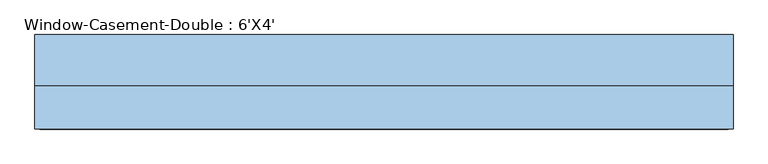
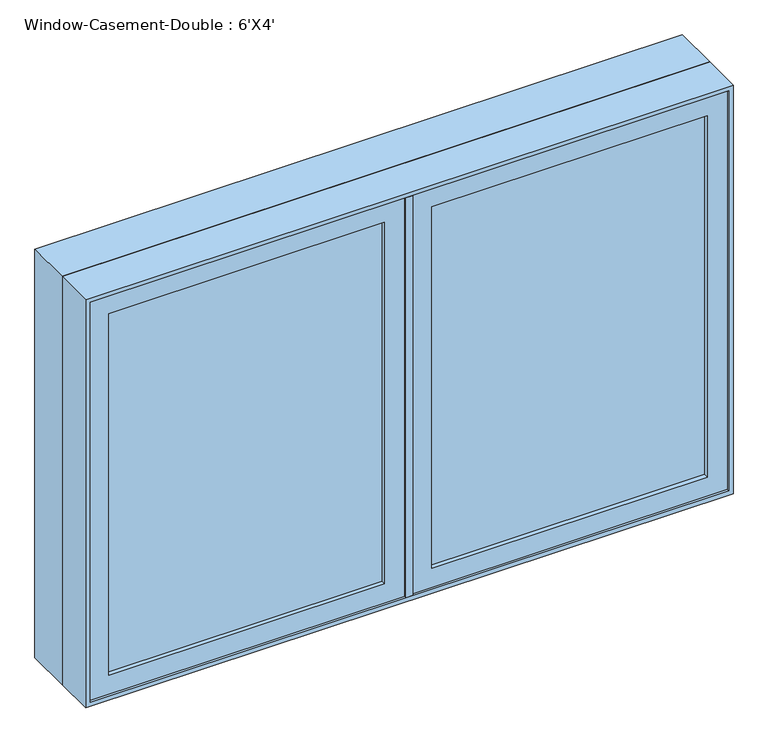
"""IFC4 building model written with IfcOpenShell, lengths in millimetres: window geometry, Window-Casement-Double : 6'X4'."""

from ifc_helpers import new_model, si_unit, frame, origin, place, context, project, spatial, polyline, outline, extrude, faceted_brep, source, transform, mapped, element, save


def window_casement_double_6_x4_44178710(model_context):
    return source(origin(), model_context, "Body", "SolidModel", [
        faceted_brep([(9.525, -133.35, 2120.9), (9.525, -82.55, 2120.9), (-9.525, -82.55, 2120.9), (-9.525, -133.35, 2120.9), (9.525, -133.35, 927.1), (-9.525, -133.35, 927.1), (-9.525, -82.55, 927.1), (9.525, -82.55, 927.1), (-9.525, -82.55, 2101.85), (-9.525, -82.55, 946.15), (-30.1625, -82.55, 2101.85), (-30.1625, -82.55, 946.15), (-30.1625, -19.05, 2101.85), (-30.1625, -19.05, 946.15), (30.1625, -19.05, 2101.85), (30.1625, -19.05, 946.15), (30.1625, -82.55, 2101.85), (30.1625, -82.55, 946.15), (9.525, -82.55, 2101.85), (9.525, -82.55, 946.15)], [[[0, 1, 2, 3]], [[4, 5, 6, 7]], [[3, 5, 4, 0]], [[2, 8, 9, 6, 5, 3]], [[8, 10, 11, 9]], [[10, 12, 13, 11]], [[12, 14, 15, 13]], [[14, 16, 17, 15]], [[16, 18, 19, 17]], [[0, 4, 7, 19, 18, 1]], [[8, 2, 1, 18]], [[19, 7, 6, 9]], [[9, 11, 13, 15, 17, 19]], [[18, 16, 14, 12, 10, 8]]]),
        extrude(outline(polyline([(-66.675, -114.3), (-844.55, -114.3), (-844.55, -107.95), (-66.675, -107.95), (-66.675, -114.3)])), frame((0.0, 0.0, 984.25), z_axis=(0.0, 0.0, 1.0), x_axis=(1.0, 0.0, 0.0)), (0.0, 0.0, 1.0), 1079.5),
        extrude(outline(polyline([(-844.55, -95.25), (-66.675, -95.25), (-66.675, -101.6), (-844.55, -101.6), (-844.55, -95.25)])), frame((0.0, 0.0, 984.25), z_axis=(0.0, 0.0, 1.0), x_axis=(1.0, 0.0, 0.0)), (0.0, 0.0, 1.0), 1079.5),
        extrude(outline(polyline([(844.55, -114.3), (66.675, -114.3), (66.675, -107.95), (844.55, -107.95), (844.55, -114.3)])), frame((0.0, 0.0, 984.25), z_axis=(0.0, 0.0, 1.0), x_axis=(1.0, 0.0, 0.0)), (0.0, 0.0, 1.0), 1079.5),
        extrude(outline(polyline([(66.675, -95.25), (844.55, -95.25), (844.55, -101.6), (66.675, -101.6), (66.675, -95.25)])), frame((0.0, 0.0, 984.25), z_axis=(0.0, 0.0, 1.0), x_axis=(1.0, 0.0, 0.0)), (0.0, 0.0, 1.0), 1079.5),
        extrude(outline(polyline([(2120.9, -9.525), (2120.9, -901.7), (927.1, -901.7), (927.1, -9.525), (2120.9, -9.525)]), holes=[polyline([(2063.75, -844.55), (2063.75, -66.675), (984.25, -66.675), (984.25, -844.55), (2063.75, -844.55)])]), frame((0.0, -127.0, 0.0), z_axis=(0.0, 1.0, 0.0), x_axis=(0.0, 0.0, 1.0)), (0.0, 0.0, 1.0), 44.45),
        extrude(outline(polyline([(927.1, 9.525), (927.1, 901.7), (2120.9, 901.7), (2120.9, 9.525), (927.1, 9.525)]), holes=[polyline([(984.25, 844.55), (984.25, 66.675), (2063.75, 66.675), (2063.75, 844.55), (984.25, 844.55)])]), frame((0.0, -127.0, 0.0), z_axis=(0.0, 1.0, 0.0), x_axis=(0.0, 0.0, 1.0)), (0.0, 0.0, 1.0), 44.45),
        extrude(outline(polyline([(2133.6, -914.4), (914.4, -914.4), (914.4, 914.4), (2133.6, 914.4), (2133.6, -914.4)]), holes=[polyline([(2114.55, 895.35), (933.45, 895.35), (933.45, -895.35), (2114.55, -895.35), (2114.55, 895.35)])]), frame((0.0, -19.05, 0.0), z_axis=(0.0, 1.0, 0.0), x_axis=(0.0, 0.0, 1.0)), (0.0, 0.0, 1.0), 133.35),
        faceted_brep([(882.65, -82.55, 2101.85), (-882.65, -82.55, 2101.85), (-882.65, -19.05, 2101.85), (882.65, -19.05, 2101.85), (901.7, -133.35, 2120.9), (-901.7, -133.35, 2120.9), (-901.7, -82.55, 2120.9), (901.7, -82.55, 2120.9), (914.4, -19.05, 2133.6), (-914.4, -19.05, 2133.6), (-914.4, -133.35, 2133.6), (914.4, -133.35, 2133.6), (-882.65, -82.55, 946.15), (-882.65, -19.05, 946.15), (-901.7, -133.35, 927.1), (-901.7, -82.55, 927.1), (-914.4, -19.05, 914.4), (-914.4, -133.35, 914.4), (882.65, -82.55, 946.15), (882.65, -19.05, 946.15), (901.7, -133.35, 927.1), (901.7, -82.55, 927.1), (914.4, -19.05, 914.4), (914.4, -133.35, 914.4)], [[[0, 1, 2, 3]], [[4, 5, 6, 7]], [[8, 9, 10, 11]], [[1, 12, 13, 2]], [[5, 14, 15, 6]], [[9, 16, 17, 10]], [[12, 18, 19, 13]], [[14, 20, 21, 15]], [[16, 22, 23, 17]], [[9, 8, 22, 16], [3, 2, 13, 19]], [[18, 0, 3, 19]], [[7, 6, 15, 21], [1, 0, 18, 12]], [[20, 4, 7, 21]], [[22, 8, 11, 23]], [[11, 10, 17, 23], [5, 4, 20, 14]]]),
    ])


if __name__ == "__main__":
    model = new_model("IFC4")
    model_context = context("Model", 3, world=origin())
    ifc_project = project(units=[si_unit("LENGTHUNIT", "METRE", prefix="MILLI")], contexts=[model_context])
    site = spatial("IfcSite", under=ifc_project)
    building = spatial("IfcBuilding", under=site)
    placement = place(None, origin())
    window_casement_double_6_x4_shape = window_casement_double_6_x4_44178710(model_context)
    element("IfcWindow", 1, ObjectType="Window-Casement-Double : 6'X4'", at=placement, inside=building, context=model_context, shape_type="MappedRepresentation", body=[
        mapped(window_casement_double_6_x4_shape, transform((0.0, 0.0, 0.0), x_axis=(1.0, 0.0, 0.0), y_axis=(0.0, 1.0, 0.0), z_axis=(0.0, 0.0, 1.0))),
    ])
    save(model, "model.ifc")

# Revit data of these elements
# Type "Window-Casement-Double : 6'X4'"
#   Type Mark = "18"
#   Fire Rating = "0.5h"
#   Assembly Code = "B2020100"
#   Analytic Construction = "Double glazing - domestic"
#   Frame Extension [instance default] = 0' - 0 1/4"
#   Window Inset [instance default] = 0' - 0"
#   Wall Thickness [instance default] = 0' - 6"
#   Interior Wall Closure [instance default] = 0' - 2 1/4"
#   Half Width = 3' - 0"
#   Visual Light Transmittance = 0.81
#   Thermal Resistance (R) = 1.8146 (h·ft²·°F)/BTU
#   Solar Heat Gain Coefficient = 0.76
#   Rough Width = 6' - 0 1/2"
#   Rough Height = 4' - 0 1/2"
#   Height = 4' - 0"
#   Heat Transfer Coefficient (U) = 0.5511 BTU/(h·ft²·°F)
#   Exterior Wall Closure [instance default] = 0' - 1 1/4"
#   Extension Jamb [instance default] = 0' - 2 1/4"
#   Default Sill Height = 3' - 0"
#   Width = 6' - 0"
#   Muntin Visibility = yes
#   Interior Trim Visibility [instance default] = yes
#   Exterior Trim Visibility [instance default] = yes
#   Extension Jamb Visibility [instance default] = yes
#   Interior Trim Material = Wood - Stained
#   Muntin Pattern = Muntin Pattern_2x2 : Muntin Pattern_2x2
#   Interior Trim = Trim-Window-Interior-Flat : Picture Frame
#   Interior Frame Material = Wood - Stained
#   Glass Panel Material = Glass
#   Exterior Trim Material = Clad - White
#   Exterior Trim = Trim-Window-Exterior-Flat : with Sill
#   Exterior Frame Material = Clad - White
#   Wall Closure = (empty or 0)
# Element 1 (IfcWindow, "Window-Casement-Double : 6'X4'")
#   Wall Thickness = 0' - 9"
#   Extension Jamb = 0' - 5 1/4"
#   Materials on its faces: "Wood - Stained", "Glass", "Clad - White"
# Materials
#   "Wood - Stained": class "Wood", colour RGB 224 178 126, transparency 0, Cost = 0
#   "Glass": class "Glass", colour RGB 0 128 192, transparency 0.75, Description = "Soda Lime Glass", Cost = 0
#   "Clad - White": class "Wood", colour RGB 242 242 238, transparency 0, Cost = 0
